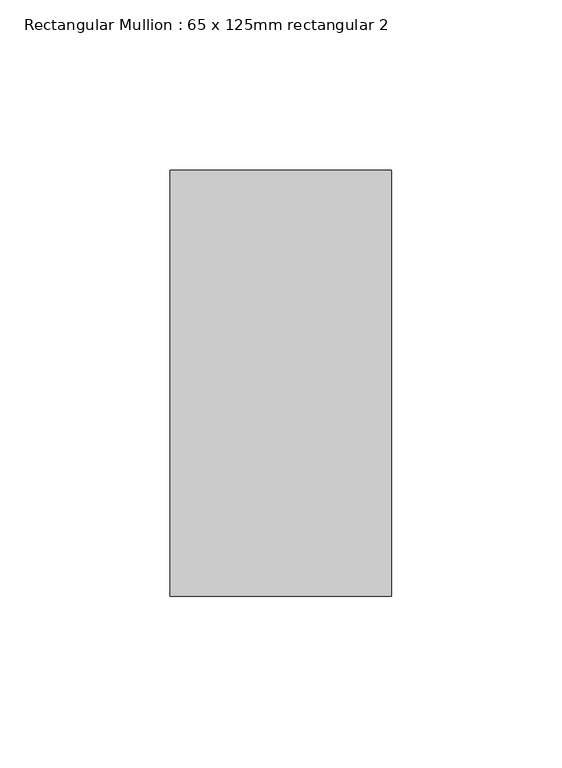
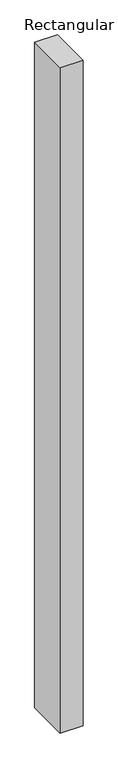
"""IFC4 building model written with IfcOpenShell, lengths in millimetres: member geometry, Rectangular Mullion : 65 x 125mm rectangular 2."""

from ifc_helpers import new_model, si_unit, frame, origin, place, context, project, spatial, polyline, outline, extrude, source, transform, mapped, element, save


def rectangular_mullion_65_x_125mm_rectangular_2_b62c991d(model_context):
    return source(origin(), model_context, "Body", "SweptSolid", [
        extrude(outline(polyline([(32.5, 62.5), (32.5, -62.5), (-32.5, -62.5), (-32.5, 62.5), (32.5, 62.5)])), frame((0.0, 0.0, -2000.0), z_axis=(0.0, 0.0, 1.0), x_axis=(1.0, 0.0, 0.0)), (0.0, 0.0, 1.0), 2000.0),
    ])


if __name__ == "__main__":
    model = new_model("IFC4")
    model_context = context("Model", 3, world=origin())
    ifc_project = project(units=[si_unit("LENGTHUNIT", "METRE", prefix="MILLI")], contexts=[model_context])
    site = spatial("IfcSite", under=ifc_project)
    building = spatial("IfcBuilding", under=site)
    placement = place(None, origin())
    rectangular_mullion_65_x_125mm_rectangular_2_shape = rectangular_mullion_65_x_125mm_rectangular_2_b62c991d(model_context)
    element("IfcMember", 1, ObjectType="Rectangular Mullion : 65 x 125mm rectangular 2", at=placement, inside=building, context=model_context, shape_type="MappedRepresentation", body=[
        mapped(rectangular_mullion_65_x_125mm_rectangular_2_shape, transform((0.0, 0.0, 0.0), x_axis=(1.0, 0.0, 0.0), y_axis=(0.0, 1.0, 0.0), z_axis=(0.0, 0.0, 1.0))),
    ])
    save(model, "model.ifc")

# Revit data of these elements
# Type "Rectangular Mullion : 65 x 125mm rectangular 2"
#   built-in parameter 1007304 = 0.410105 (stored number, unit not read)
#   built-in parameter 1007301 = 0.106627 (stored number, unit not read)
#   built-in parameter 1007300 = 0.106627 (stored number, unit not read)
